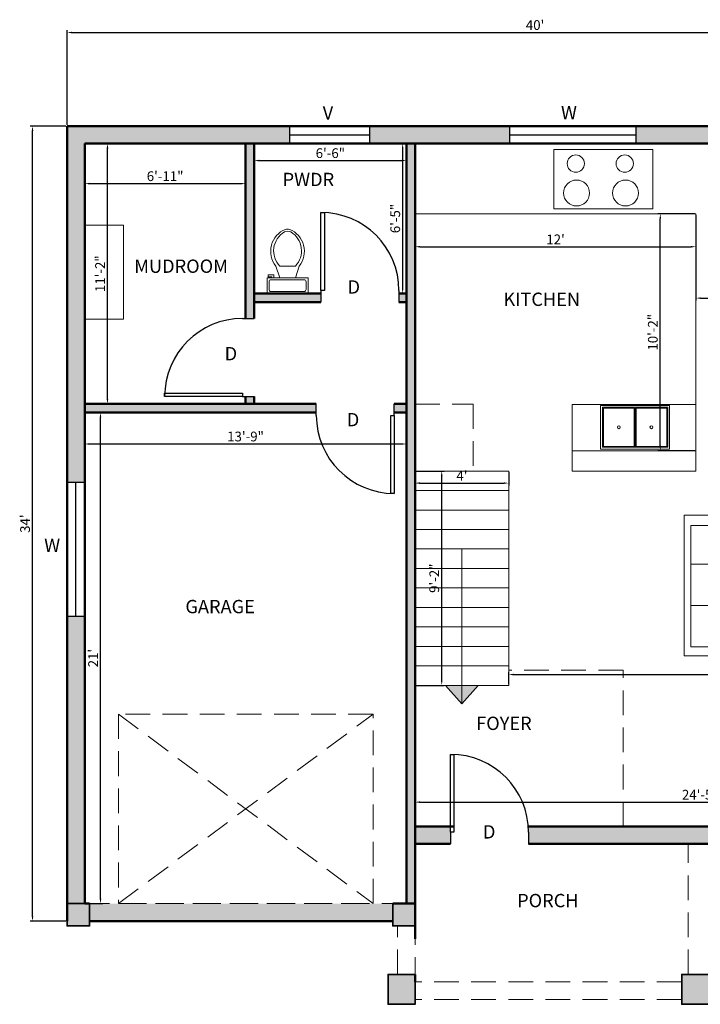
# Model space of a CAD drawing. Units: inches. Extents: x 1838 to 3464, y 573 to 2547.
# Tile 2 of 6: x 2100 to 2449, y 1302 to 1808. Entities that reach past the tile are written whole.
import ezdxf

# ---------------------------------------------------------------- set-up
doc = ezdxf.new("R2010")
doc.units = ezdxf.units.IN
doc.linetypes.add('DASHED', pattern=[19.05, 12.7, -6.35])
for name, color, linetype, lineweight in [('A-ANNO-DIMS', 2, 'Continuous', 18), ('A-ANNO-TEXT', 7, 'Continuous', 18), ('A-AREA-IDEN', 3, 'Continuous', 18), ('A-COLS', 6, 'Continuous', 35), ('A-DOOR', 4, 'Continuous', 25), ('A-FLOR-FIXT', 9, 'Continuous', 18), ('A-FLOR-OVHD', 8, 'DASHED', 18), ('A-FLOR-STRS', 2, 'Continuous', 18), ('A-FURN', 8, 'Continuous', 18), ('A-GLAZ', 3, 'Continuous', 25), ('A-WALL', 1, 'Continuous', 50), ('A-WALL-PATT', 8, 'Continuous', 13)]:
    doc.layers.add(name, color=color, linetype=linetype, lineweight=lineweight)
doc.styles.get("Standard").update_dxf_attribs({"font": 'arial.ttf'})
doc.dimstyles.new('ISO-25', dxfattribs={"dimtxt": 5, "dimasz": 2.5, "dimexe": 1.25, "dimexo": 0.625, "dimtad": 1, "dimdec": 0, "dimlunit": 4, "dimtxsty": 'Standard', "dimcen": 2.5, "dimadec": 0, "dimazin": 0, "dimtfac": 1, "dimtdec": 0, "dimtmove": 0, "dimatfit": 3, "dimfxl": 1, "dimarcsym": 0})

# ---------------------------------------------------------------- blocks, each defined once
blk = doc.blocks.new('*U2')
for p, q in [((0, 0), (0, -6)), ((40, 0), (40, -6))]:
    blk.add_line(p, q)
blk.add_lwpolyline([(0, 0), (0, 40), (1.75, 40), (1.75, 0)], close=True)
blk.add_arc((0, 0), 40, 0, 90)
blk = doc.blocks.new('*U4')
for p, q in [((9.5, -6), (9.5, -2)), ((-10, -8.5), (-8, -8.5)), ((-10, -9.5), (-10, -8.5)), ((-7, -9.5), (-10, -9.5)), ((-8, -8.5), (-8, -8)), ((-7, -8), (-7, -9.5)), ((-4, -8), (-6, -14)), ((4, -8), (6, -14)), ((4, -14), (-4, -14))]:
    blk.add_line(p, q)
blk.add_lwpolyline([(10.5, -8), (10.5, 0), (-10.5, 0), (-10.5, -8)], close=True)
for points in [[(-9.5, -2), (-9.5, -6)], [(8.5, -1), (-8.5, -1)], [(-8.5, -7), (8.5, -7)]]:
    blk.add_lwpolyline(points)
for centre, radius, start, end in [((-8.62, -1.88), 0.884, 81.8699, 188.1301), ((8.62, -1.88), 0.884, 351.8699, 98.1301), ((-8.62, -6.12), 0.884, 171.8699, 278.1301), ((8.62, -6.12), 0.884, 261.8699, 8.1301), ((3.52, -21.58), 12.17, 141.4691, 247.9714), ((4.2, -21.82), 11.33, 136.3677, 238.9468), ((-3.52, -21.58), 12.17, 292.0284, 38.5307), ((-4.2, -21.82), 11.33, 301.053, 43.6321), ((0, -27.88), 4, 245.7318, 294.2682), ((0, -29), 4, 254.8605, 285.1395)]:
    blk.add_arc(centre, radius, start, end)
blk = doc.blocks.new('*D7')
at = {"layer": 'A-ANNO-DIMS', "color": 0, "lineweight": -2, "transparency": 16777216}
for p, q in [((2133.46, 1743.46), (2133.46, 1722.32)), ((2215.96, 1743.46), (2215.96, 1722.32)), ((2135.96, 1723.57), (2213.46, 1723.57))]:
    blk.add_line(p, q, dxfattribs=at)
at = {"layer": 'A-ANNO-DIMS', "color": 0, "lineweight": 100, "transparency": 16777216}
for points in [[(2135.96, 1723.99), (2135.96, 1723.16), (2133.46, 1723.57)], [(2213.46, 1723.99), (2213.46, 1723.16), (2215.96, 1723.57)]]:
    blk.add_solid(points, dxfattribs=at)
at = {"layer": 'Defpoints', "color": 0, "lineweight": 100, "transparency": 16777216}
for p in [(2133.46, 1744.09), (2215.96, 1744.09), (2215.96, 1723.57)]:
    blk.add_point(p, dxfattribs=at)
at = {"layer": 'A-ANNO-DIMS', "color": 0, "transparency": 16777216, "insert": (2174.71, 1726.75), "char_height": 5, "attachment_point": 5}
blk.add_mtext('6\'-11"', dxfattribs=at)
blk = doc.blocks.new('*D8')
at = {"layer": 'A-ANNO-DIMS', "color": 0, "lineweight": -2, "transparency": 16777216}
for p, q in [((2134.08, 1744.09), (2146.4, 1744.09)), ((2145.15, 1613.09), (2145.15, 1741.59)), ((2134.08, 1610.59), (2146.4, 1610.59))]:
    blk.add_line(p, q, dxfattribs=at)
at = {"layer": 'A-ANNO-DIMS', "color": 0, "lineweight": 100, "transparency": 16777216}
for points in [[(2144.73, 1741.59), (2145.57, 1741.59), (2145.15, 1744.09)], [(2144.73, 1613.09), (2145.57, 1613.09), (2145.15, 1610.59)]]:
    blk.add_solid(points, dxfattribs=at)
at = {"layer": 'Defpoints', "color": 0, "lineweight": 100, "transparency": 16777216}
for p in [(2133.46, 1744.09), (2145.15, 1744.09), (2133.46, 1610.59)]:
    blk.add_point(p, dxfattribs=at)
at = {"layer": 'A-ANNO-DIMS', "color": 0, "transparency": 16777216, "insert": (2142.01, 1677.34), "char_height": 5, "attachment_point": 5, "rotation": 90}
blk.add_mtext('11\'-2"', dxfattribs=at)
blk = doc.blocks.new('*D9')
at = {"layer": 'A-ANNO-DIMS', "color": 0, "lineweight": -2, "transparency": 16777216}
for p, q in [((2220.46, 1743.46), (2220.46, 1734.15)), ((2298.46, 1743.46), (2298.46, 1734.15)), ((2222.96, 1735.4), (2295.96, 1735.4))]:
    blk.add_line(p, q, dxfattribs=at)
at = {"layer": 'A-ANNO-DIMS', "color": 0, "lineweight": 100, "transparency": 16777216}
for points in [[(2222.96, 1735.82), (2222.96, 1734.98), (2220.46, 1735.4)], [(2295.96, 1735.82), (2295.96, 1734.98), (2298.46, 1735.4)]]:
    blk.add_solid(points, dxfattribs=at)
at = {"layer": 'Defpoints', "color": 0, "lineweight": 100, "transparency": 16777216}
for p in [(2220.46, 1744.09), (2298.46, 1744.09), (2298.46, 1735.4)]:
    blk.add_point(p, dxfattribs=at)
at = {"layer": 'A-ANNO-DIMS', "color": 0, "transparency": 16777216, "insert": (2259.46, 1738.58), "char_height": 5, "attachment_point": 5}
blk.add_mtext('6\'-6"', dxfattribs=at)
blk = doc.blocks.new('*D10')
at = {"layer": 'A-ANNO-DIMS', "color": 0, "lineweight": -2, "transparency": 16777216}
for p, q in [((2297.83, 1744.09), (2295.3, 1744.09)), ((2296.55, 1741.59), (2296.55, 1669.76)), ((2297.83, 1667.26), (2295.3, 1667.26))]:
    blk.add_line(p, q, dxfattribs=at)
at = {"layer": 'A-ANNO-DIMS', "color": 0, "lineweight": 100, "transparency": 16777216}
for points in [[(2296.14, 1741.59), (2296.97, 1741.59), (2296.55, 1744.09)], [(2296.14, 1669.76), (2296.97, 1669.76), (2296.55, 1667.26)]]:
    blk.add_solid(points, dxfattribs=at)
at = {"layer": 'Defpoints', "color": 0, "lineweight": 100, "transparency": 16777216}
for p in [(2298.46, 1744.09), (2296.55, 1667.26), (2298.46, 1667.26)]:
    blk.add_point(p, dxfattribs=at)
at = {"layer": 'A-ANNO-DIMS', "color": 0, "transparency": 16777216, "insert": (2293.38, 1705.67), "char_height": 5, "attachment_point": 5, "rotation": 90}
blk.add_mtext('6\'-5"', dxfattribs=at)
blk = doc.blocks.new('*D11')
at = {"layer": 'A-ANNO-DIMS', "color": 0, "lineweight": -2, "transparency": 16777216}
for p, q in [((2133.46, 1605.46), (2133.46, 1588.72)), ((2298.46, 1605.46), (2298.46, 1588.72)), ((2135.96, 1589.97), (2295.96, 1589.97))]:
    blk.add_line(p, q, dxfattribs=at)
at = {"layer": 'A-ANNO-DIMS', "color": 0, "lineweight": 100, "transparency": 16777216}
for points in [[(2135.96, 1590.38), (2135.96, 1589.55), (2133.46, 1589.97)], [(2295.96, 1590.38), (2295.96, 1589.55), (2298.46, 1589.97)]]:
    blk.add_solid(points, dxfattribs=at)
at = {"layer": 'Defpoints', "color": 0, "lineweight": 100, "transparency": 16777216}
for p in [(2133.46, 1606.09), (2298.46, 1606.09), (2298.46, 1589.97)]:
    blk.add_point(p, dxfattribs=at)
at = {"layer": 'A-ANNO-DIMS', "color": 0, "transparency": 16777216, "insert": (2215.96, 1593.15), "char_height": 5, "attachment_point": 5}
blk.add_mtext('13\'-9"', dxfattribs=at)
blk = doc.blocks.new('*D12')
at = {"layer": 'A-ANNO-DIMS', "color": 0, "lineweight": -2, "transparency": 16777216}
for p, q in [((2134.08, 1606.09), (2142.82, 1606.09)), ((2141.57, 1356.59), (2141.57, 1603.59)), ((2134.08, 1354.09), (2142.82, 1354.09))]:
    blk.add_line(p, q, dxfattribs=at)
at = {"layer": 'A-ANNO-DIMS', "color": 0, "lineweight": 100, "transparency": 16777216}
for points in [[(2141.15, 1603.59), (2141.98, 1603.59), (2141.57, 1606.09)], [(2141.15, 1356.59), (2141.98, 1356.59), (2141.57, 1354.09)]]:
    blk.add_solid(points, dxfattribs=at)
at = {"layer": 'Defpoints', "color": 0, "lineweight": 100, "transparency": 16777216}
for p in [(2133.46, 1606.09), (2141.57, 1606.09), (2133.46, 1354.09)]:
    blk.add_point(p, dxfattribs=at)
at = {"layer": 'A-ANNO-DIMS', "color": 0, "transparency": 16777216, "insert": (2138.43, 1480.09), "char_height": 5, "attachment_point": 5, "rotation": 90}
blk.add_mtext("21'", dxfattribs=at)
blk = doc.blocks.new('*D13')
at = {"layer": 'A-ANNO-DIMS', "color": 0, "lineweight": -2, "transparency": 16777216}
for p, q in [((2302.96, 1394.32), (2302.96, 1407.41)), ((2305.46, 1406.16), (2592.96, 1406.16)), ((2595.46, 1394.32), (2595.46, 1407.41))]:
    blk.add_line(p, q, dxfattribs=at)
at = {"layer": 'A-ANNO-DIMS', "color": 0, "lineweight": 100, "transparency": 16777216}
for points in [[(2305.46, 1406.58), (2305.46, 1405.75), (2302.96, 1406.16)], [(2592.96, 1406.58), (2592.96, 1405.75), (2595.46, 1406.16)]]:
    blk.add_solid(points, dxfattribs=at)
at = {"layer": 'Defpoints', "color": 0, "lineweight": 100, "transparency": 16777216}
for p in [(2595.46, 1406.16), (2302.96, 1393.69), (2595.46, 1393.69)]:
    blk.add_point(p, dxfattribs=at)
at = {"layer": 'A-ANNO-DIMS', "color": 0, "transparency": 16777216, "insert": (2449.21, 1409.34), "char_height": 5, "attachment_point": 5}
blk.add_mtext('24\'-5"', dxfattribs=at)
blk = doc.blocks.new('*D16')
at = {"layer": 'A-ANNO-DIMS', "color": 0, "lineweight": -2, "transparency": 16777216}
for p, q in [((2446.96, 1707.46), (2446.96, 1663.58)), ((2595.46, 1707.46), (2595.46, 1663.58)), ((2449.46, 1664.83), (2592.96, 1664.83))]:
    blk.add_line(p, q, dxfattribs=at)
at = {"layer": 'A-ANNO-DIMS', "color": 0, "lineweight": 100, "transparency": 16777216}
for points in [[(2449.46, 1665.25), (2449.46, 1664.41), (2446.96, 1664.83)], [(2592.96, 1665.25), (2592.96, 1664.41), (2595.46, 1664.83)]]:
    blk.add_solid(points, dxfattribs=at)
at = {"layer": 'Defpoints', "color": 0, "lineweight": 100, "transparency": 16777216}
for p in [(2446.96, 1708.09), (2595.46, 1708.09), (2595.46, 1664.83)]:
    blk.add_point(p, dxfattribs=at)
at = {"layer": 'A-ANNO-DIMS', "color": 0, "transparency": 16777216, "insert": (2521.21, 1668.01), "char_height": 5, "attachment_point": 5}
blk.add_mtext('12\'-5"', dxfattribs=at)
blk = doc.blocks.new('*D17')
at = {"layer": 'A-ANNO-DIMS', "color": 0, "lineweight": -2, "transparency": 16777216}
for p, q in [((2350.96, 1466.71), (2350.96, 1472.89)), ((2353.46, 1471.64), (2583.23, 1471.64)), ((2585.73, 1466.71), (2585.73, 1472.89))]:
    blk.add_line(p, q, dxfattribs=at)
at = {"layer": 'A-ANNO-DIMS', "color": 0, "lineweight": 100, "transparency": 16777216}
for points in [[(2353.46, 1472.06), (2353.46, 1471.23), (2350.96, 1471.64)], [(2583.23, 1472.06), (2583.23, 1471.23), (2585.73, 1471.64)]]:
    blk.add_solid(points, dxfattribs=at)
at = {"layer": 'Defpoints', "color": 0, "lineweight": 100, "transparency": 16777216}
for p in [(2585.73, 1471.64), (2350.96, 1466.09), (2585.73, 1466.09)]:
    blk.add_point(p, dxfattribs=at)
at = {"layer": 'A-ANNO-DIMS', "color": 0, "transparency": 16777216, "insert": (2468.34, 1474.82), "char_height": 5, "attachment_point": 5}
blk.add_mtext('19\'-7"', dxfattribs=at)
blk = doc.blocks.new('*D18')
at = {"layer": 'A-ANNO-DIMS', "color": 0, "lineweight": -2, "transparency": 16777216}
for p, q in [((2302.96, 1575.46), (2302.96, 1568.64)), ((2350.96, 1575.46), (2350.96, 1568.64)), ((2305.46, 1569.89), (2348.46, 1569.89))]:
    blk.add_line(p, q, dxfattribs=at)
at = {"layer": 'A-ANNO-DIMS', "color": 0, "lineweight": 100, "transparency": 16777216}
for points in [[(2305.46, 1570.31), (2305.46, 1569.47), (2302.96, 1569.89)], [(2348.46, 1570.31), (2348.46, 1569.47), (2350.96, 1569.89)]]:
    blk.add_solid(points, dxfattribs=at)
at = {"layer": 'Defpoints', "color": 0, "lineweight": 100, "transparency": 16777216}
for p in [(2302.96, 1576.09), (2350.96, 1576.09), (2350.96, 1569.89)]:
    blk.add_point(p, dxfattribs=at)
at = {"layer": 'A-ANNO-DIMS', "color": 0, "transparency": 16777216, "insert": (2326.96, 1573.02), "char_height": 5, "attachment_point": 5}
blk.add_mtext("4'", dxfattribs=at)
blk = doc.blocks.new('*D19')
at = {"layer": 'A-ANNO-DIMS', "color": 0, "lineweight": -2, "transparency": 16777216}
for p, q in [((2303.58, 1576.09), (2317.83, 1576.09)), ((2316.58, 1468.59), (2316.58, 1573.59)), ((2303.58, 1466.09), (2317.83, 1466.09))]:
    blk.add_line(p, q, dxfattribs=at)
at = {"layer": 'A-ANNO-DIMS', "color": 0, "lineweight": 100, "transparency": 16777216}
for points in [[(2316.16, 1573.59), (2316.99, 1573.59), (2316.58, 1576.09)], [(2316.16, 1468.59), (2316.99, 1468.59), (2316.58, 1466.09)]]:
    blk.add_solid(points, dxfattribs=at)
at = {"layer": 'Defpoints', "color": 0, "lineweight": 100, "transparency": 16777216}
for p in [(2302.96, 1576.09), (2316.58, 1576.09), (2302.96, 1466.09)]:
    blk.add_point(p, dxfattribs=at)
at = {"layer": 'A-ANNO-DIMS', "color": 0, "transparency": 16777216, "insert": (2313.4, 1521.09), "char_height": 5, "attachment_point": 5, "rotation": 90}
blk.add_mtext('9\'-2"', dxfattribs=at)
blk = doc.blocks.new('*D20')
at = {"layer": 'A-ANNO-DIMS', "color": 0, "lineweight": -2, "transparency": 16777216}
for p, q in [((2124.46, 1753.71), (2124.46, 1802.37)), ((2126.96, 1801.12), (2601.96, 1801.12)), ((2604.46, 1753.71), (2604.46, 1802.37))]:
    blk.add_line(p, q, dxfattribs=at)
at = {"layer": 'A-ANNO-DIMS', "color": 0, "lineweight": 100, "transparency": 16777216}
for points in [[(2126.96, 1801.54), (2126.96, 1800.7), (2124.46, 1801.12)], [(2601.96, 1801.54), (2601.96, 1800.7), (2604.46, 1801.12)]]:
    blk.add_solid(points, dxfattribs=at)
at = {"layer": 'Defpoints', "color": 0, "lineweight": 100, "transparency": 16777216}
for p in [(2604.46, 1801.12), (2124.46, 1753.09), (2604.46, 1753.09)]:
    blk.add_point(p, dxfattribs=at)
at = {"layer": 'A-ANNO-DIMS', "color": 0, "transparency": 16777216, "insert": (2364.46, 1804.3), "char_height": 5, "attachment_point": 5}
blk.add_mtext("40'", dxfattribs=at)
blk = doc.blocks.new('*D21')
at = {"layer": 'A-ANNO-DIMS', "color": 0, "lineweight": -2, "transparency": 16777216}
for p, q in [((2123.83, 1753.09), (2105.47, 1753.09)), ((2106.72, 1347.59), (2106.72, 1750.59)), ((2123.83, 1345.09), (2105.47, 1345.09))]:
    blk.add_line(p, q, dxfattribs=at)
at = {"layer": 'A-ANNO-DIMS', "color": 0, "lineweight": 100, "transparency": 16777216}
for points in [[(2106.3, 1750.59), (2107.13, 1750.59), (2106.72, 1753.09)], [(2106.3, 1347.59), (2107.13, 1347.59), (2106.72, 1345.09)]]:
    blk.add_solid(points, dxfattribs=at)
at = {"layer": 'Defpoints', "color": 0, "lineweight": 100, "transparency": 16777216}
for p in [(2106.72, 1753.09), (2124.46, 1753.09), (2124.46, 1345.09)]:
    blk.add_point(p, dxfattribs=at)
at = {"layer": 'A-ANNO-DIMS', "color": 0, "transparency": 16777216, "insert": (2103.54, 1549.09), "char_height": 5, "attachment_point": 5, "rotation": 90}
blk.add_mtext("34'", dxfattribs=at)
blk = doc.blocks.new('*D63')
at = {"layer": 'A-ANNO-DIMS', "color": 0, "lineweight": -2, "transparency": 16777216}
for p, q in [((2302.96, 1707.46), (2302.96, 1689.93)), ((2446.96, 1707.46), (2446.96, 1689.93)), ((2305.46, 1691.18), (2444.46, 1691.18))]:
    blk.add_line(p, q, dxfattribs=at)
at = {"layer": 'A-ANNO-DIMS', "color": 0, "lineweight": 100, "transparency": 16777216}
for points in [[(2305.46, 1691.59), (2305.46, 1690.76), (2302.96, 1691.18)], [(2444.46, 1691.59), (2444.46, 1690.76), (2446.96, 1691.18)]]:
    blk.add_solid(points, dxfattribs=at)
at = {"layer": 'Defpoints', "color": 0, "lineweight": 100, "transparency": 16777216}
for p in [(2302.96, 1708.09), (2446.96, 1708.09), (2446.96, 1691.18)]:
    blk.add_point(p, dxfattribs=at)
at = {"layer": 'A-ANNO-DIMS', "color": 0, "transparency": 16777216, "insert": (2374.96, 1694.31), "char_height": 5, "attachment_point": 5}
blk.add_mtext("12'", dxfattribs=at)
blk = doc.blocks.new('*D64')
at = {"layer": 'A-ANNO-DIMS', "color": 0, "lineweight": -2, "transparency": 16777216}
for p, q in [((2446.33, 1708.09), (2427.43, 1708.09)), ((2428.68, 1589.02), (2428.68, 1705.59)), ((2446.33, 1586.52), (2427.43, 1586.52))]:
    blk.add_line(p, q, dxfattribs=at)
at = {"layer": 'A-ANNO-DIMS', "color": 0, "lineweight": 100, "transparency": 16777216}
for points in [[(2428.27, 1705.59), (2429.1, 1705.59), (2428.68, 1708.09)], [(2428.27, 1589.02), (2429.1, 1589.02), (2428.68, 1586.52)]]:
    blk.add_solid(points, dxfattribs=at)
at = {"layer": 'Defpoints', "color": 0, "lineweight": 100, "transparency": 16777216}
for p in [(2428.68, 1708.09), (2446.96, 1708.09), (2446.96, 1586.52)]:
    blk.add_point(p, dxfattribs=at)
at = {"layer": 'A-ANNO-DIMS', "color": 0, "transparency": 16777216, "insert": (2425.51, 1647.3), "char_height": 5, "attachment_point": 5, "rotation": 90}
blk.add_mtext('10\'-2"', dxfattribs=at)

msp = doc.modelspace()

# ---------------------------------------------------------------- hatches: boundary and pattern name
at = {"layer": 'A-FLOR-STRS'}
h = msp.add_hatch(color=256, dxfattribs=at)
h.dxf.hatch_style = 1
h.paths.add_polyline_path([(2326.96, 1466.09), (2318.55, 1466.09), (2326.96, 1456.6)])
h.paths.add_polyline_path([(2335.36, 1466.09), (2326.96, 1466.09), (2326.96, 1456.6)])
at = {"layer": 'A-WALL-PATT'}
h = msp.add_hatch(color=256, dxfattribs=at)
h.dxf.hatch_style = 1
h.paths.add_polyline_path([(2238.51, 1753.09), (2124.46, 1753.09), (2124.46, 1570.41), (2133.46, 1570.41), (2133.46, 1606.09), (2133.46, 1744.09), (2238.51, 1744.09)])
h.paths.add_polyline_path([(2351.42, 1753.09), (2279.74, 1753.09), (2279.74, 1744.09), (2351.42, 1744.09)])
h.paths.add_polyline_path([(2503.16, 1753.09), (2416.24, 1753.09), (2416.24, 1744.09), (2446.96, 1744.09), (2503.16, 1744.09)])
h.paths.add_polyline_path([(2604.46, 1753.09), (2565.42, 1753.09), (2565.42, 1744.09), (2595.46, 1744.09), (2595.46, 1683.21), (2604.46, 1683.21)])
h.paths.add_polyline_path([(2133.46, 1501.38), (2124.46, 1501.38), (2124.46, 1354.09), (2133.46, 1354.09)])
h.paths.add_polyline_path([(2291.43, 1354.09), (2135.98, 1354.09), (2135.98, 1345.09), (2291.43, 1345.09)])
h.paths.add_polyline_path([(2321.13, 1390.69), (2321.13, 1393.69), (2302.96, 1393.69), (2302.96, 1384.69), (2321.13, 1384.69)])
h.paths.add_polyline_path([(2482.67, 1393.69), (2361.02, 1393.69, -0.01877), (2361.13, 1390.69), (2361.13, 1384.69), (2482.67, 1384.69)])
h.paths.add_polyline_path([(2302.96, 1576.09), (2302.96, 1610.48), (2302.96, 1744.09), (2298.46, 1744.09), (2298.46, 1571.59), (2298.46, 1354.09), (2302.96, 1354.09)])
h.paths.add_polyline_path([(2595.46, 1393.69), (2566.49, 1393.69), (2566.49, 1384.69), (2595.46, 1384.69)])
h.paths.add_polyline_path([(2604.46, 1526.49), (2595.46, 1526.49), (2595.46, 1404.09), (2595.46, 1384.69), (2604.46, 1384.69)])
h.paths.add_polyline_path([(2604.46, 1614.19), (2595.46, 1614.19), (2595.46, 1595.51), (2604.46, 1595.51)])
h = msp.add_hatch(color=256, dxfattribs=at)
h.dxf.hatch_style = 1
h.paths.add_polyline_path([(2220.46, 1744.09), (2215.96, 1744.09), (2215.96, 1654.37), (2220.46, 1654.37)])
h.paths.add_polyline_path([(2254.65, 1667.26), (2220.46, 1667.26), (2220.46, 1662.76), (2254.65, 1662.76)])
h.paths.add_polyline_path([(2298.46, 1667.26), (2294.65, 1667.26), (2294.65, 1662.76), (2298.46, 1662.76)])
h.paths.add_polyline_path([(2252.26, 1610.59), (2133.46, 1610.59), (2133.46, 1606.09), (2252.26, 1606.09)])
h.paths.add_polyline_path([(2298.46, 1610.59), (2292.26, 1610.59), (2292.26, 1606.09), (2298.46, 1606.09)])
h.paths.add_polyline_path([(2220.46, 1614.37), (2215.96, 1614.37), (2215.96, 1610.59), (2220.46, 1610.59)])
h = msp.add_hatch(color=256, dxfattribs=at)
h.dxf.hatch_style = 1
h.paths.add_polyline_path([(2135.98, 1354.09), (2124.46, 1354.09), (2124.46, 1342.67), (2135.98, 1342.67)])
h.paths.add_polyline_path([(2302.96, 1354.09), (2291.43, 1354.09), (2291.43, 1342.67), (2302.96, 1342.67)])
h.paths.add_polyline_path([(2453.5, 1317.8), (2439.65, 1317.8), (2439.65, 1302.42), (2453.5, 1302.42)])
h.paths.add_polyline_path([(2302.96, 1317.8), (2289.1, 1317.8), (2289.1, 1302.42), (2302.96, 1302.42)])
h.paths.add_polyline_path([(2604.33, 1317.8), (2590.48, 1317.8), (2590.48, 1302.42), (2604.33, 1302.42)])

# ---------------------------------------------------------------- linework, layer by layer
at = {"layer": 'A-COLS'}
for points in [[(2135.98, 1354.09), (2124.46, 1354.09), (2124.46, 1342.67), (2135.98, 1342.67)], [(2302.96, 1354.09), (2291.43, 1354.09), (2291.43, 1342.67), (2302.96, 1342.67)], [(2302.96, 1317.8), (2289.1, 1317.8), (2289.1, 1302.42), (2302.96, 1302.42)], [(2453.5, 1317.8), (2439.65, 1317.8), (2439.65, 1302.42), (2453.5, 1302.42)]]:
    msp.add_lwpolyline(points, close=True, dxfattribs=at)
msp.add_lwpolyline([(2289.1, 1345.09), (2291.43, 1345.09)], dxfattribs=at)
at = {"layer": 'A-FLOR-FIXT'}
for p, q in [((2302.96, 1708.09), (2446.96, 1708.09)), ((2446.96, 1708.09), (2446.96, 1576.09)), ((2415.75, 1588.25), (2415.75, 1608.78)), ((2383.55, 1586.52), (2446.96, 1586.52)), ((2446.96, 1576.09), (2383.55, 1576.09)), ((2383.55, 1576.09), (2446.96, 1576.09))]:
    msp.add_line(p, q, dxfattribs=at)
for points in [[(2374.12, 1710.57), (2424.94, 1710.57), (2424.94, 1741.14), (2374.12, 1741.14)], [(2446.96, 1576.09), (2383.55, 1576.09), (2383.55, 1610.24), (2446.96, 1610.24)], [(2398.02, 1587.25), (2433.49, 1587.25), (2433.49, 1609.78), (2398.02, 1609.78)], [(2399.02, 1588.25), (2432.49, 1588.25), (2432.49, 1608.78), (2399.02, 1608.78)], [(2399.02, 1588.25), (2415.75, 1588.25), (2415.75, 1608.78), (2399.02, 1608.78)], [(2399.52, 1588.75), (2415.25, 1588.75), (2415.25, 1608.28), (2399.52, 1608.28)], [(2415.75, 1588.25), (2432.49, 1588.25), (2432.49, 1608.78), (2415.75, 1608.78)], [(2416.25, 1588.75), (2431.99, 1588.75), (2431.99, 1608.28), (2416.25, 1608.28)]]:
    msp.add_lwpolyline(points, close=True, dxfattribs=at)
for centre, radius in [((2385.35, 1733.85), 4.43), ((2410.47, 1733.85), 4.43), ((2385.76, 1718.76), 6.65), ((2410.87, 1718.76), 6.65), ((2407.39, 1598.52), 0.726), ((2424.12, 1598.52), 0.726)]:
    msp.add_circle(centre, radius, dxfattribs=at)
at = {"layer": 'A-FLOR-OVHD'}
for p, q in [((2409.63, 1473.93), (2350.96, 1473.93)), ((2409.63, 1393.69), (2409.63, 1473.93)), ((2150.75, 1354.09), (2281.36, 1451.32)), ((2150.75, 1451.32), (2281.36, 1354.09)), ((2443, 1317.8), (2443, 1384.69)), ((2133.46, 1354.09), (2291.43, 1354.09)), ((2293.96, 1317.8), (2293.96, 1342.67)), ((2302.96, 1313.93), (2302.96, 1336.01)), ((2439.65, 1313.93), (2302.96, 1313.93)), ((2439.65, 1304.93), (2302.96, 1304.93))]:
    msp.add_line(p, q, dxfattribs=at)
for points in [[(2302.96, 1610.48), (2332.71, 1610.48), (2332.71, 1576.09), (2302.96, 1576.09)], [(2150.75, 1354.09), (2281.36, 1354.09), (2281.36, 1451.32), (2150.75, 1451.32)]]:
    msp.add_lwpolyline(points, close=True, dxfattribs=at)
at = {"layer": 'A-FLOR-STRS'}
for p, q in [((2302.96, 1576.09), (2350.96, 1576.09)), ((2350.96, 1571.59), (2350.96, 1576.09)), ((2350.96, 1466.09), (2350.96, 1571.59)), ((2302.96, 1566.09), (2350.96, 1566.09)), ((2302.96, 1556.09), (2350.96, 1556.09)), ((2302.96, 1546.09), (2350.96, 1546.09)), ((2302.96, 1536.09), (2350.96, 1536.09)), ((2326.96, 1466.09), (2326.96, 1536.09)), ((2326.96, 1536.09), (2326.96, 1456.6)), ((2302.96, 1526.09), (2350.96, 1526.09)), ((2302.96, 1516.09), (2350.96, 1516.09)), ((2302.96, 1506.09), (2350.96, 1506.09)), ((2302.96, 1496.09), (2350.96, 1496.09)), ((2302.96, 1486.09), (2350.96, 1486.09)), ((2302.96, 1476.09), (2350.96, 1476.09)), ((2302.96, 1466.09), (2350.96, 1466.09)), ((2326.96, 1456.6), (2318.55, 1466.09)), ((2326.96, 1456.6), (2335.36, 1466.09))]:
    msp.add_line(p, q, dxfattribs=at)
at = {"layer": 'A-FURN'}
for p, q in [((2441.01, 1481.22), (2441.01, 1553.46)), ((2441.01, 1553.46), (2466.28, 1553.46)), ((2469.8, 1528.32), (2444.27, 1528.32)), ((2469.8, 1507.14), (2444.27, 1507.14)), ((2466.28, 1481.22), (2441.01, 1481.22))]:
    msp.add_line(p, q, dxfattribs=at)
for points in [[(2133.46, 1654.01), (2153.41, 1654.01), (2153.41, 1702.2), (2133.46, 1702.2)], [(2469.8, 1548.22), (2444.27, 1548.22), (2444.27, 1485.82), (2469.8, 1485.82)]]:
    msp.add_lwpolyline(points, close=True, dxfattribs=at)
at = {"layer": 'A-GLAZ'}
for p, q in [((2238.51, 1748.59), (2279.74, 1748.59)), ((2351.42, 1748.59), (2416.24, 1748.59)), ((2128.96, 1501.38), (2128.96, 1570.41))]:
    msp.add_line(p, q, dxfattribs=at)
for points in [[(2238.51, 1744.09), (2279.74, 1744.09), (2279.74, 1753.09), (2238.51, 1753.09)], [(2351.42, 1744.09), (2416.24, 1744.09), (2416.24, 1753.09), (2351.42, 1753.09)], [(2124.46, 1570.41), (2133.46, 1570.41), (2133.46, 1501.38), (2124.46, 1501.38)]]:
    msp.add_lwpolyline(points, close=True, dxfattribs=at)
at = {"layer": 'A-WALL'}
for p, q in [((2124.46, 1753.09), (2604.46, 1753.09)), ((2124.46, 1345.09), (2124.46, 1753.09)), ((2133.46, 1744.09), (2595.46, 1744.09)), ((2133.46, 1354.09), (2133.46, 1744.09)), ((2215.96, 1654.37), (2215.96, 1744.09)), ((2220.46, 1654.37), (2220.46, 1744.09)), ((2298.46, 1744.09), (2298.46, 1571.59)), ((2446.96, 1744.09), (2302.96, 1744.09)), ((2302.96, 1744.09), (2302.96, 1576.09)), ((2302.96, 1744.09), (2302.96, 1720.09)), ((2220.46, 1667.26), (2254.65, 1667.26)), ((2220.46, 1662.76), (2254.65, 1662.76)), ((2294.65, 1667.26), (2298.46, 1667.26)), ((2294.65, 1662.76), (2298.46, 1662.76)), ((2215.96, 1610.59), (2215.96, 1614.37)), ((2220.46, 1610.59), (2220.46, 1614.37)), ((2133.46, 1610.59), (2252.26, 1610.59)), ((2292.26, 1610.59), (2298.46, 1610.59)), ((2133.46, 1354.09), (2133.46, 1606.09)), ((2133.46, 1606.09), (2252.26, 1606.09)), ((2292.26, 1606.09), (2298.46, 1606.09)), ((2298.46, 1571.59), (2298.46, 1354.09)), ((2302.96, 1576.09), (2302.96, 1354.09)), ((2322.88, 1393.69), (2302.96, 1393.69)), ((2595.46, 1393.69), (2361.02, 1393.69)), ((2321.13, 1384.69), (2302.96, 1384.69)), ((2595.46, 1384.69), (2361.13, 1384.69)), ((2135.98, 1354.09), (2133.46, 1354.09)), ((2302.96, 1354.09), (2291.43, 1354.09)), ((2302.96, 1354.09), (2302.96, 1345.09)), ((2291.43, 1345.09), (2135.98, 1345.09)), ((2302.96, 1345.09), (2302.96, 1336.01)), ((2302.96, 1317.8), (2302.96, 1313.93))]:
    msp.add_line(p, q, dxfattribs=at)
msp.add_lwpolyline([(2302.96, 1345.09), (2302.96, 1336.01)], dxfattribs=at)

# ---------------------------------------------------------------- block references
at = {"layer": 'A-DOOR'}
for p in [(2254.65, 1668.76), (2321.13, 1390.69)]:
    msp.add_blockref('*U2', p, dxfattribs=at)
for p, rotation in [((2214.46, 1614.37), 90), ((2292.26, 1604.59), 180)]:
    msp.add_blockref('*U2', p, dxfattribs=dict(at, rotation=rotation))
at = {"layer": 'A-FLOR-FIXT', "xscale": -1, "rotation": 180}
msp.add_blockref('*U4', (2237.51, 1667.26), dxfattribs=at)

# ---------------------------------------------------------------- texts
at = {"layer": 'A-ANNO-TEXT', "char_height": 6.84, "attachment_point": 1}
for s, insert in [('W', (2377.74, 1763.47)), ('V', (2255.55, 1763.28)), ('D', (2268.29, 1673.98)), ('D', (2205.25, 1639.73)), ('D', (2267.89, 1605.87)), ('W', (2112.68, 1541.42)), ('D', (2337.73, 1394.35))]:
    msp.add_mtext_dynamic_manual_height_columns(s, width=95.5762, gutter_width=34.2, heights=[0], dxfattribs=dict(at, insert=insert))
at = {"layer": 'A-AREA-IDEN', "char_height": 6.841, "attachment_point": 1}
for s, insert in [('PWDR', (2234.97, 1729.13)), ('MUDROOM', (2158.86, 1684.63)), ('KITCHEN', (2348.19, 1667.65)), ('GARAGE', (2185.11, 1509.95)), ('FOYER', (2334.26, 1450.04)), ('PORCH', (2355.26, 1359.08))]:
    msp.add_mtext_dynamic_manual_height_columns(s, width=95.5762, gutter_width=34.2, heights=[0], dxfattribs=dict(at, insert=insert))

# ---------------------------------------------------------------- dimensions: what is measured, and where the dimension line sits
at = {"layer": 'A-ANNO-DIMS'}
for base, p1, p2, picture, middle in [((2604.46, 1801.12), (2124.46, 1753.09), (2604.46, 1753.09), '*D20', (2364.46, 1804.3)), ((2215.95522311, 1723.57317222), (2133.45522311, 1744.08520436), (2215.95522311, 1744.08520436), '*D7', (2174.70522311, 1726.75103716)), ((2298.46, 1735.4), (2220.46, 1744.09), (2298.46, 1744.09), '*D9', (2259.46, 1738.58)), ((2446.96, 1691.18), (2302.96, 1708.09), (2446.96, 1708.09), '*D63', (2374.96, 1694.31)), ((2595.45522311, 1664.82921857), (2446.95522311, 1708.08520436), (2595.45522311, 1708.08520436), '*D16', (2521.20522311, 1668.00708351)), ((2298.46, 1589.97), (2133.46, 1606.09), (2298.46, 1606.09), '*D11', (2215.96, 1593.15)), ((2350.96, 1569.89), (2302.96, 1576.09), (2350.96, 1576.09), '*D18', (2326.96, 1573.02)), ((2585.73, 1471.64), (2350.96, 1466.09), (2585.73, 1466.09), '*D17', (2468.34, 1474.82)), ((2595.45522311, 1406.16307805), (2302.95522311, 1393.69353478), (2595.45522311, 1393.69353478), '*D13', (2449.20522311, 1409.34094299))]:
    dim = msp.add_linear_dim(base=base, p1=p1, p2=p2, dimstyle='ISO-25', override={"dimclrd": 0, "dimclre": 0, "dimclrt": 0}, dxfattribs=at)
    dim.commit()
    dim.dimension.update_dxf_attribs({"geometry": picture, "text_midpoint": middle})
for base, p1, p2, picture, middle in [((2106.72, 1753.09), (2124.46, 1345.09), (2124.46, 1753.09), '*D21', (2103.54, 1549.09)), ((2145.1496609, 1744.08520436), (2133.45522311, 1610.58520436), (2133.45522311, 1744.08520436), '*D8', (2142.01442897, 1677.33520436)), ((2296.55, 1667.26), (2298.46, 1744.09), (2298.46, 1667.26), '*D10', (2293.38, 1705.67)), ((2428.68, 1708.09), (2446.96, 1586.52), (2446.96, 1708.09), '*D64', (2425.51, 1647.3)), ((2141.57, 1606.09), (2133.46, 1354.09), (2133.46, 1606.09), '*D12', (2138.43, 1480.09)), ((2316.58, 1576.09), (2302.96, 1466.09), (2302.96, 1576.09), '*D19', (2313.4, 1521.09))]:
    dim = msp.add_linear_dim(base=base, p1=p1, p2=p2, angle=90, dimstyle='ISO-25', override={"dimclrd": 0, "dimclre": 0, "dimclrt": 0}, dxfattribs=at)
    dim.commit()
    dim.dimension.update_dxf_attribs({"geometry": picture, "text_midpoint": middle})

doc.saveas('drawing.dxf')
